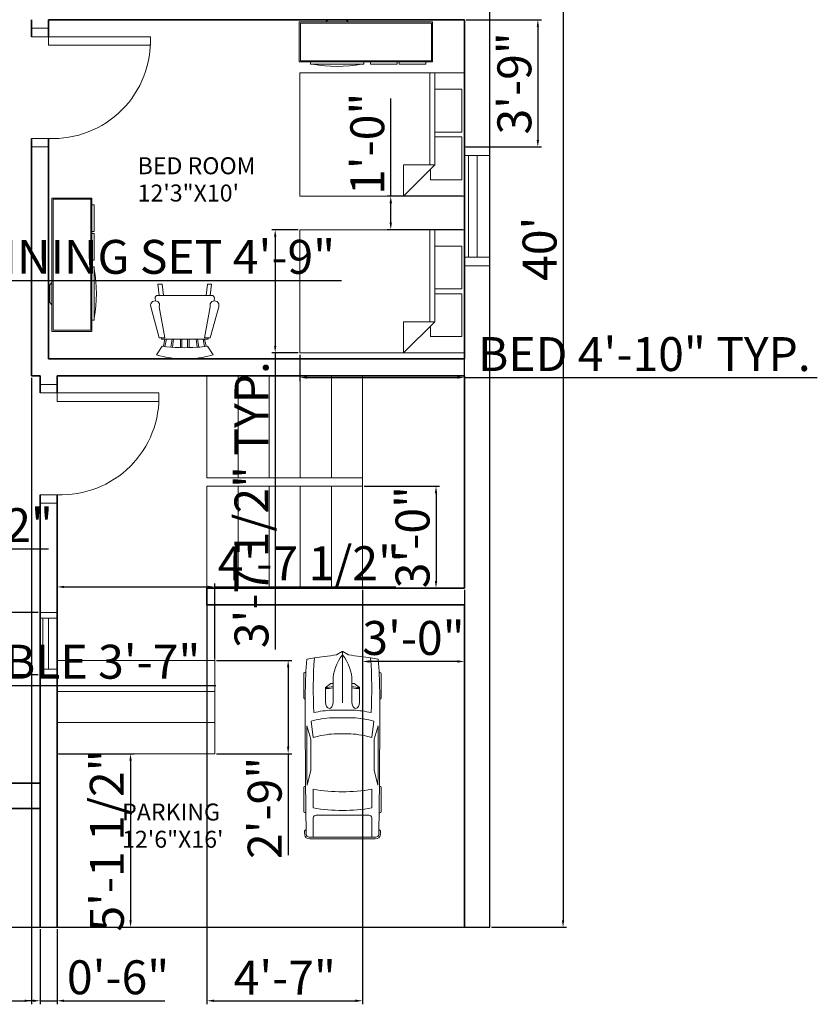
# Model space of a CAD drawing. Units: inches. Extents: x 2021 to 2692, y 429 to 1061.
# Tile 4 of 5: x 2362 to 2644, y 480 to 828. Entities that reach past the tile are written whole.
import ezdxf

# ---------------------------------------------------------------- set-up
doc = ezdxf.new("R2010")
doc.units = ezdxf.units.IN
for name, color, linetype, lineweight in [('A-ANNO-DIMS', 2, 'Continuous', 18), ('A-AREA-IDEN', 7, 'Continuous', 18), ('A-DOOR', 4, 'Continuous', 18), ('A-FLOR-STRS', 7, 'Continuous', 18), ('A-FURN', 8, 'Continuous', 13), ('A-GLAZ', 4, 'Continuous', 18), ('A-WALL', 7, 'Continuous', 35), ('C-PRKG-VEHI', 8, 'Continuous', 13), ('C-PROP', 3, 'Continuous', 25)]:
    doc.layers.add(name, color=color, linetype=linetype, lineweight=lineweight)
doc.styles.get("Standard").update_dxf_attribs({"font": 'arial.ttf'})
doc.dimstyles.new('ISO-25', dxfattribs={"dimtxt": 12, "dimasz": 2.5, "dimexe": 1.25, "dimexo": 0.625, "dimtad": 1, "dimdec": 0, "dimlunit": 3, "dimtxsty": 'Standard', "dimcen": 2.5, "dimadec": 0, "dimazin": 0, "dimtfac": 1, "dimtdec": 0, "dimtmove": 0, "dimatfit": 3, "dimfxl": 1, "dimarcsym": 0})

# ---------------------------------------------------------------- blocks, each defined once
blk = doc.blocks.new('Bed - Queen')
for p, q in [((0, -80.00003), (0, 0)), ((0, 0), (59.99999, 0)), ((59.99999, 0), (59.99999, -80.00003)), ((7.99999, -1.2), (28.79998, -1.2)), ((7.99999, -14.4), (7.99999, -1.2)), ((28.79998, -1.2), (28.79998, -14.4)), ((31.19999, -1.2), (51.99999, -1.2)), ((31.19999, -14.4), (31.19999, -1.2)), ((51.99999, -1.2), (51.99999, -16.4)), ((0, -14.4), (44.8, -14.4)), ((44.8, -16.8), (0, -16.8)), ((59.99999, -29.6), (44.8, -14.4)), ((44.8, -14.4), (44.8, -29.6)), ((51.99999, -16.4), (46.79936, -16.4)), ((44.8, -29.6), (59.99999, -29.6)), ((59.99999, -80.00003), (0, -80.00003))]:
    blk.add_line(p, q)
blk = doc.blocks.new('Entertainment Center')
for p, q in [((-4, 0), (-5, -1)), ((4, 0), (-4, 0)), ((5, -1), (4, 0)), ((-17, -19), (-17, -1)), ((-17, -1), (43, -1)), ((-16.5, -18.5), (-16.5, -1.5)), ((-16.5, -1.5), (42.5, -1.5)), ((42.5, -1.5), (42.5, -18.5)), ((43, -1), (43, -19)), ((43, -19), (-17, -19)), ((42.5, -18.5), (-16.5, -18.5)), ((-12, -20), (-12, -19)), ((12, -20), (-12, -20)), ((12, -19), (12, -20)), ((15, -20), (15, -19)), ((27, -20), (15, -20)), ((27, -19), (27, -20)), ((28, -20), (28, -19)), ((40, -20), (28, -20)), ((40, -19), (40, -20))]:
    blk.add_line(p, q)
blk.add_arc((0, 40), 61, 259.6111, 280.3889)
blk = doc.blocks.new('Chair - Rocking')
for p, q in [((-8, -4.5), (-10, -1.5)), ((8, -4.5), (10, -1.5)), ((-7.5, -4.5), (-7, -7)), ((-6.5, -7), (-7.02225, -4.43)), ((-4.5, -7), (-4.96674, -4.19951)), ((-4, -7), (-4.40532, -4.16272)), ((-1.5, -4.05012), (-1.5, -7)), ((-1, -7), (-1, -4.05012)), ((1, -7), (1, -4.04655)), ((1.5, -4.05012), (1.5, -7)), ((4, -7), (4.40187, -4.18694)), ((4.5, -7), (4.96761, -4.19437)), ((6.5, -7), (7, -4.4057)), ((7.5, -4.5), (7, -7)), ((-9, -7.5), (-12, -18.49999)), ((-7, -7.5), (-9, -7.5)), ((-9, -18.49999), (-7, -7.5)), ((-8.23428, -6.99939), (-8.3093, -7.47958)), ((-8.23041, -7), (8.23915, -7)), ((7, -7.5), (9, -7.5)), ((9, -18.49999), (7, -7.5)), ((8.31071, -7.48854), (8.23449, -7.00073)), ((9, -7.5), (12, -18.49999)), ((-10.36644, -20.64523), (-10.5, -21.49999)), ((10.5, -21.49999), (10.3575, -20.58798)), ((-9, -22.49999), (-9.5, -26.49999)), ((0, -22.49999), (-9.5, -22.49999)), ((-8, -26.49999), (-7.5, -22.49999)), ((0, -22.49999), (9.5, -22.49999)), ((8, -26.49999), (7.5, -22.49999)), ((9, -22.49999), (9.5, -26.49999)), ((-9.5, -26.49999), (-8, -26.49999)), ((9.5, -26.49999), (8, -26.49999))]:
    blk.add_line(p, q)
for centre, radius, start, end in [((0, -34.08333), 34.08333, 72.93847, 107.0615), ((0, -68.25004), 64.25, 93.92211, 97.15267), ((0, -68.25004), 64.25, 82.84733, 93.92211), ((-10.5, -18.99999), 1.58114, 161.5651, 18.43495), ((10.5, -18.99999), 1.58114, 161.5651, 18.43495), ((-9.5, -21.49999), 1, 180, 270), ((9.5, -21.49999), 1, 270, 0)]:
    blk.add_arc(centre, radius, start, end)
blk = doc.blocks.new('*U14')
for p, q in [((21.1, 37.41), (21.1, 36.83)), ((46.55, 38.89), (22.35, 38.89)), ((47.8, 37.39), (47.8, 37.41)), ((70.03, 31.54), (86.41, 29.35)), ((87.99, 31.87), (74.76, 35.92)), ((134.31, 35.6), (119.29, 31.78)), ((135.45, 37.07), (135.45, 37.41)), ((136.7, 38.89), (160.9, 38.89)), ((162.15, 37.41), (162.15, 36.77)), ((186.47, -33.5), (186.47, 33.5)), ((188.4, -32.76), (188.4, 32.76)), ((138.42, 29.35), (157.25, 29.35)), ((164.52, 26.39), (164.52, -26.39)), ((186.47, 29.35), (167.01, 29.35)), ((32.12, 9.51), (32.12, 11.15)), ((32.27, 11.63), (36.13, 17.17)), ((36.13, 17.17), (50.94, 17.17)), ((58.92, -10.77), (58.92, 10.77)), ((66.55, -10.53), (66.55, 10.53)), ((186.47, -10.53), (186.47, 10.53)), ((3.27, 6.13), (0.1, 0.41)), ((29.77, 9.51), (51.68, 9.51)), ((82.74, 8.5), (82.74, -8.5)), ((0, 0), (51.68, 0)), ((0.1, -0.41), (3.27, -6.13)), ((29.77, -9.51), (51.68, -9.51)), ((32.12, -9.51), (32.12, -11.15)), ((32.27, -11.63), (36.13, -17.17)), ((36.13, -17.17), (50.94, -17.17)), ((86.41, -29.35), (70.03, -31.54)), ((157.25, -29.35), (138.42, -29.35)), ((167.01, -29.35), (186.47, -29.35)), ((21.1, -37.41), (21.1, -36.83)), ((46.55, -38.89), (22.35, -38.89)), ((47.8, -37.39), (47.8, -37.41)), ((87.99, -31.87), (74.76, -35.92)), ((134.31, -35.6), (119.29, -31.78)), ((135.45, -37.07), (135.45, -37.41)), ((136.7, -38.89), (160.9, -38.89)), ((162.15, -37.41), (162.15, -36.77))]:
    blk.add_line(p, q)
for centre, major_axis, ratio, start_param, end_param in [((266.03, -27.52), (0, 313.31), 0.842304, 1.367076, 1.39176), ((37.47, -593.96), (0, -623.33), 0.842304, 3.096046, 3.200911), ((41.19, -490.86), (0, 528.23), 0.842304, 0.00281, 0.075598), ((22.35, 37.41), (0, -1.48), 0.842304, 3.141593, 4.712389), ((64.48, -10555.62), (0, 10593.03), 0.842304, -0.013397, 0.002797), ((46.55, 37.41), (0, 1.48), 0.842304, -1.570796, 0), ((135.29, 5.39), (0, 81.77), 0.842304, 1.245306, 1.50788), ((64.48, -10555.62), (0, -10591.55), 0.842304, 3.133765, 3.140441), ((95.79, -3666.35), (0, -3698.24), 0.842304, 3.134049, 3.144098), ((136.7, 37.41), (0, -1.48), 0.842304, 3.141593, 4.712389), ((160.9, 37.41), (0, 1.48), 0.842304, -1.570796, 0), ((180.63, 35.84), (0, 2.22), 0.842304, -0.013017, 1.249894), ((64.48, -10556.36), (0, 10595.31), 0.842304, -0.013397, -0.013017), ((183.98, 33.5), (0, -2.96), 0.842304, 1.570796, 3.128196), ((183.98, 32.76), (0, -5.25), 0.842304, 1.570796, 3.128196), ((259.18, -27.52), (0, -305.3), 0.842304, 4.528606, 4.561838), ((134.4, 5.39), (0, -89.78), 0.842304, 4.449482, 4.652344), ((149.6, 2.8), (0, -79.58), 0.842304, 4.372215, 4.640744), ((17.08, 0), (0, 147.02), 0.842304, 4.511394, 4.913384), ((35.91, 0), (0, 147.02), 0.842304, 4.511394, 4.913384), ((167.01, 26.39), (0, 2.96), 0.842304, 0, 1.570796), ((-204.49, 52.4), (0, -250.96), 0.842304, 1.385369, 1.434372), ((32.75, 11.15), (0, 0.74), 0.842304, 0.879714, 1.570796), ((13.04, 17.01), (0, 27.42), 0.842304, 4.435146, 4.718221), ((14.2, 17.01), (0, 27.42), 0.842304, 4.435146, 4.718221), ((50.79, 13.34), (6.34, -0.36), 0.603834, -1.395552, 1.581315), ((0.62, 0), (0, -0.74), 0.842304, 4.131459, 5.293319), ((29.77, -46.66), (0, 56.17), 0.842304, 0, 0.590319), ((-204.49, -52.4), (0, 250.96), 0.842304, -1.434372, -1.385369), ((29.77, 46.66), (0, 56.17), 0.842304, 2.551274, 3.141593), ((13.04, -17.01), (0, -27.42), 0.842304, 1.564964, 1.848039), ((14.2, -17.01), (0, -27.42), 0.842304, 1.564964, 1.848039), ((149.6, -2.8), (0, -79.58), 0.842304, -1.499151, -1.230623), ((259.18, 27.52), (0, 305.3), 0.842304, 1.721348, 1.754579), ((32.75, -11.15), (0, -0.74), 0.842304, 4.712389, 5.403472), ((134.4, -5.39), (0, -89.78), 0.842304, -1.510751, -1.307889), ((135.29, -5.39), (0, -81.77), 0.842304, -1.50788, -1.245306), ((266.03, 27.52), (0, 313.31), 0.842304, 1.749832, 1.774517), ((37.47, 593.96), (0, -623.33), 0.842304, -0.059319, 0.045547), ((167.01, -26.39), (0, -2.96), 0.842304, 4.712389, 6.283185), ((41.19, 490.86), (0, -528.23), 0.842304, -0.075598, -0.00281), ((22.35, -37.41), (0, 1.48), 0.842304, 1.570796, 3.141593), ((64.48, 10555.62), (0, 10593.03), 0.842304, 3.138796, 3.15499), ((46.55, -37.41), (0, -1.48), 0.842304, 0, 1.570796), ((64.48, 10555.62), (0, -10591.55), 0.842304, 0.001152, 0.007828), ((95.79, 3666.35), (0, -3698.24), 0.842304, -0.002505, 0.007544), ((136.7, -37.41), (0, -1.48), 0.842304, -1.570796, 0), ((160.9, -37.41), (0, 1.48), 0.842304, 3.141593, 4.712389), ((180.63, -35.84), (0, -2.22), 0.842304, -1.249894, 0.013017), ((64.48, 10556.36), (0, 10595.31), 0.842304, 3.15461, 3.15499), ((183.98, -33.5), (0, 2.96), 0.842304, 3.15499, 4.712389), ((183.98, -32.76), (0, -5.25), 0.842304, 0.013397, 1.570796)]:
    blk.add_ellipse(centre, major_axis=major_axis, ratio=ratio, start_param=start_param, end_param=end_param)
at = {"extrusion": (0, 0, -1)}
blk.add_ellipse((50.79, -13.34), major_axis=(6.34, 0.36), ratio=0.603834, start_param=-1.395552, end_param=1.581315, dxfattribs=at)
blk = doc.blocks.new('*D16')
at = {"layer": 'A-ANNO-DIMS', "color": 0, "lineweight": -2, "transparency": 16777216}
for p, q in [((2528.73, 986.96), (2555.26, 986.96)), ((2554.01, 984.46), (2554.01, 509.46)), ((2528.73, 506.96), (2555.26, 506.96))]:
    blk.add_line(p, q, dxfattribs=at)
at = {"layer": 'A-ANNO-DIMS', "color": 0, "transparency": 16777216}
for points in [[(2553.59, 984.46), (2554.43, 984.46), (2554.01, 986.96)], [(2553.59, 509.46), (2554.43, 509.46), (2554.01, 506.96)]]:
    blk.add_solid(points, dxfattribs=at)
at = {"layer": 'Defpoints', "color": 0, "transparency": 16777216}
for p in [(2528.11, 986.96), (2528.11, 506.96), (2554.01, 506.96)]:
    blk.add_point(p, dxfattribs=at)
at = {"layer": 'A-ANNO-DIMS', "color": 0, "transparency": 16777216, "insert": (2547.26, 746.96), "char_height": 12, "attachment_point": 5, "rotation": 90}
blk.add_mtext("40'", dxfattribs=at)
blk = doc.blocks.new('DOOR-SWING-36IN')
for p, q in [((36.03, 42), (42.03, 42)), ((36.03, 39), (42.03, 39)), ((36.03, 3), (42.03, 3)), ((36.03, 0), (42.03, 0))]:
    blk.add_line(p, q)
blk.add_lwpolyline([(36.03, 39), (0.03, 39), (0.03, 36), (36.03, 36)], close=True)
blk.add_arc((34.53, 37.5), 34.53, 177.5104, 272.4896)
blk = doc.blocks.new('WIN-36IN')
for p, q in [((0, 0), (0, 9)), ((3, 9), (39, 9)), ((3, 0), (3, 9)), ((3, 7.5), (39, 7.5)), ((39, 9), (39, 0)), ((42, 9), (42, 0)), ((3, 4.5), (39, 4.5)), ((39, 0), (3, 0))]:
    blk.add_line(p, q)
blk = doc.blocks.new('*D28')
at = {"layer": 'A-ANNO-DIMS', "color": 0, "lineweight": -2, "transparency": 16777216}
for p, q in [((2460.96, 709.49), (2460.96, 700.15)), ((2519.08, 709.49), (2519.08, 700.15)), ((2463.46, 701.4), (2516.58, 701.4)), ((2519.08, 701.4), (2643.89, 701.4))]:
    blk.add_line(p, q, dxfattribs=at)
at = {"layer": 'A-ANNO-DIMS', "color": 0, "transparency": 16777216}
for points in [[(2463.46, 701.81), (2463.46, 700.98), (2460.96, 701.4)], [(2516.58, 701.81), (2516.58, 700.98), (2519.08, 701.4)]]:
    blk.add_solid(points, dxfattribs=at)
at = {"layer": 'Defpoints', "color": 0, "transparency": 16777216}
for p in [(2460.96, 710.11), (2519.08, 710.11), (2519.08, 701.4)]:
    blk.add_point(p, dxfattribs=at)
at = {"layer": 'A-ANNO-DIMS', "color": 0, "transparency": 16777216, "insert": (2582.73, 708.15), "char_height": 12, "attachment_point": 5}
blk.add_mtext('BED 4\'-10" TYP.', dxfattribs=at)
blk = doc.blocks.new('*D29')
at = {"layer": 'A-ANNO-DIMS', "color": 0, "lineweight": -2, "transparency": 16777216}
for p, q in [((2460.33, 753.7), (2450.99, 753.7)), ((2452.24, 751.2), (2452.24, 712.61)), ((2460.33, 710.11), (2450.99, 710.11)), ((2452.24, 710.11), (2452.24, 605.27))]:
    blk.add_line(p, q, dxfattribs=at)
at = {"layer": 'A-ANNO-DIMS', "color": 0, "transparency": 16777216}
for points in [[(2451.82, 751.2), (2452.65, 751.2), (2452.24, 753.7)], [(2451.82, 712.61), (2452.65, 712.61), (2452.24, 710.11)]]:
    blk.add_solid(points, dxfattribs=at)
at = {"layer": 'Defpoints', "color": 0, "transparency": 16777216}
for p in [(2460.96, 753.7), (2452.24, 710.11), (2460.96, 710.11)]:
    blk.add_point(p, dxfattribs=at)
at = {"layer": 'A-ANNO-DIMS', "color": 0, "transparency": 16777216, "insert": (2445.4, 656.44), "char_height": 12, "attachment_point": 5, "rotation": 90}
blk.add_mtext('3\'-7 1/2" TYP.', dxfattribs=at)
blk = doc.blocks.new('*D38')
at = {"layer": 'A-ANNO-DIMS', "color": 0, "lineweight": -2, "transparency": 16777216}
for p, q in [((2283.11, 743.62), (2283.11, 734.45)), ((2340.09, 743.62), (2340.09, 734.45)), ((2285.61, 735.7), (2337.59, 735.7)), ((2340.09, 735.7), (2475.73, 735.7))]:
    blk.add_line(p, q, dxfattribs=at)
at = {"layer": 'A-ANNO-DIMS', "color": 0, "transparency": 16777216}
for points in [[(2285.61, 736.12), (2285.61, 735.28), (2283.11, 735.7)], [(2337.59, 736.12), (2337.59, 735.28), (2340.09, 735.7)]]:
    blk.add_solid(points, dxfattribs=at)
at = {"layer": 'Defpoints', "color": 0, "transparency": 16777216}
for p in [(2283.11, 744.25), (2340.09, 744.25), (2340.09, 735.7)]:
    blk.add_point(p, dxfattribs=at)
at = {"layer": 'A-ANNO-DIMS', "color": 0, "transparency": 16777216, "insert": (2409.16, 742.53), "char_height": 12, "attachment_point": 5}
blk.add_mtext('DINING SET 4\'-9"', dxfattribs=at)
blk = doc.blocks.new('*D47')
at = {"layer": 'A-ANNO-DIMS', "color": 0, "lineweight": -2, "transparency": 16777216}
for p, q in [((2278.74, 634.19), (2278.74, 642.06)), ((2281.24, 640.81), (2305.76, 640.81)), ((2308.26, 634.19), (2308.26, 642.06)), ((2308.26, 640.81), (2372.08, 640.81))]:
    blk.add_line(p, q, dxfattribs=at)
at = {"layer": 'A-ANNO-DIMS', "color": 0, "transparency": 16777216}
for points in [[(2281.24, 641.23), (2281.24, 640.4), (2278.74, 640.81)], [(2305.76, 641.23), (2305.76, 640.4), (2308.26, 640.81)]]:
    blk.add_solid(points, dxfattribs=at)
at = {"layer": 'Defpoints', "color": 0, "transparency": 16777216}
for p in [(2308.26, 640.81), (2278.74, 633.57), (2308.26, 633.57)]:
    blk.add_point(p, dxfattribs=at)
at = {"layer": 'A-ANNO-DIMS', "color": 0, "transparency": 16777216, "insert": (2341.42, 647.64), "char_height": 12, "attachment_point": 5}
blk.add_mtext('2\'-5 1/2"', dxfattribs=at)
blk = doc.blocks.new('*D48')
at = {"layer": 'A-ANNO-DIMS', "color": 0, "lineweight": -2, "transparency": 16777216}
for p, q in [((2222.09, 598.36), (2222.09, 591.25)), ((2265.33, 598.36), (2265.33, 591.25)), ((2224.59, 592.5), (2262.83, 592.5)), ((2265.33, 592.5), (2431.25, 592.5))]:
    blk.add_line(p, q, dxfattribs=at)
at = {"layer": 'A-ANNO-DIMS', "color": 0, "transparency": 16777216}
for points in [[(2224.59, 592.92), (2224.59, 592.08), (2222.09, 592.5)], [(2262.83, 592.92), (2262.83, 592.08), (2265.33, 592.5)]]:
    blk.add_solid(points, dxfattribs=at)
at = {"layer": 'Defpoints', "color": 0, "transparency": 16777216}
for p in [(2222.09, 598.99), (2265.33, 598.99), (2265.33, 592.5)]:
    blk.add_point(p, dxfattribs=at)
at = {"layer": 'A-ANNO-DIMS', "color": 0, "transparency": 16777216, "insert": (2349.54, 599.34), "char_height": 12, "attachment_point": 5}
blk.add_mtext('COFFEE TABLE 3\'-7"', dxfattribs=at)
blk = doc.blocks.new('*D55')
at = {"layer": 'A-ANNO-DIMS', "color": 0, "lineweight": -2, "transparency": 16777216}
for p, q in [((2369.11, 506.34), (2369.11, 479.73)), ((2375.11, 506.34), (2375.11, 479.73)), ((2366.61, 480.98), (2364.11, 480.98)), ((2369.11, 480.98), (2375.11, 480.98)), ((2377.61, 480.98), (2413.26, 480.98))]:
    blk.add_line(p, q, dxfattribs=at)
at = {"layer": 'A-ANNO-DIMS', "color": 0, "transparency": 16777216}
for points in [[(2366.61, 481.4), (2366.61, 480.56), (2369.11, 480.98)], [(2377.61, 481.4), (2377.61, 480.56), (2375.11, 480.98)]]:
    blk.add_solid(points, dxfattribs=at)
at = {"layer": 'Defpoints', "color": 0, "transparency": 16777216}
for p in [(2369.11, 506.96), (2375.11, 506.96), (2375.11, 480.98)]:
    blk.add_point(p, dxfattribs=at)
at = {"layer": 'A-ANNO-DIMS', "color": 0, "transparency": 16777216, "insert": (2396.68, 487.73), "char_height": 12, "attachment_point": 5}
blk.add_mtext('0\'-6"', dxfattribs=at)
blk = doc.blocks.new('*D56')
at = {"layer": 'A-ANNO-DIMS', "color": 0, "lineweight": -2, "transparency": 16777216}
for p, q in [((2375.11, 601.99), (2375.11, 628.6)), ((2377.61, 627.35), (2428.34, 627.35)), ((2430.84, 601.99), (2430.84, 628.6)), ((2430.84, 627.35), (2494.93, 627.35))]:
    blk.add_line(p, q, dxfattribs=at)
at = {"layer": 'A-ANNO-DIMS', "color": 0, "transparency": 16777216}
for points in [[(2377.61, 627.77), (2377.61, 626.94), (2375.11, 627.35)], [(2428.34, 627.77), (2428.34, 626.94), (2430.84, 627.35)]]:
    blk.add_solid(points, dxfattribs=at)
at = {"layer": 'Defpoints', "color": 0, "transparency": 16777216}
for p in [(2430.84, 627.35), (2375.11, 601.37), (2430.84, 601.37)]:
    blk.add_point(p, dxfattribs=at)
at = {"layer": 'A-ANNO-DIMS', "color": 0, "transparency": 16777216, "insert": (2464.13, 634.18), "char_height": 12, "attachment_point": 5}
blk.add_mtext('4\'-7 1/2"', dxfattribs=at)
blk = doc.blocks.new('*D57')
at = {"layer": 'A-ANNO-DIMS', "color": 0, "lineweight": -2, "transparency": 16777216}
for p, q in [((2431.46, 601.37), (2458.07, 601.37)), ((2456.82, 598.87), (2456.82, 570.87)), ((2431.46, 568.37), (2458.07, 568.37)), ((2456.82, 568.37), (2456.82, 532.52))]:
    blk.add_line(p, q, dxfattribs=at)
at = {"layer": 'A-ANNO-DIMS', "color": 0, "transparency": 16777216}
for points in [[(2456.41, 598.87), (2457.24, 598.87), (2456.82, 601.37)], [(2456.41, 570.87), (2457.24, 570.87), (2456.82, 568.37)]]:
    blk.add_solid(points, dxfattribs=at)
at = {"layer": 'Defpoints', "color": 0, "transparency": 16777216}
for p in [(2430.84, 601.37), (2430.84, 568.37), (2456.82, 568.37)]:
    blk.add_point(p, dxfattribs=at)
at = {"layer": 'A-ANNO-DIMS', "color": 0, "transparency": 16777216, "insert": (2450.07, 549.19), "char_height": 12, "attachment_point": 5, "rotation": 90}
blk.add_mtext('2\'-9"', dxfattribs=at)
blk = doc.blocks.new('*D58')
at = {"layer": 'A-ANNO-DIMS', "color": 0, "lineweight": -2, "transparency": 16777216}
for p, q in [((2483.73, 662.96), (2510.34, 662.96)), ((2509.09, 660.46), (2509.09, 629.46)), ((2483.73, 626.96), (2510.34, 626.96))]:
    blk.add_line(p, q, dxfattribs=at)
at = {"layer": 'A-ANNO-DIMS', "color": 0, "transparency": 16777216}
for points in [[(2508.68, 660.46), (2509.51, 660.46), (2509.09, 662.96)], [(2508.68, 629.46), (2509.51, 629.46), (2509.09, 626.96)]]:
    blk.add_solid(points, dxfattribs=at)
at = {"layer": 'Defpoints', "color": 0, "transparency": 16777216}
for p in [(2483.11, 662.96), (2483.11, 626.96), (2509.09, 626.96)]:
    blk.add_point(p, dxfattribs=at)
at = {"layer": 'A-ANNO-DIMS', "color": 0, "transparency": 16777216, "insert": (2502.34, 644.96), "char_height": 12, "attachment_point": 5, "rotation": 90}
blk.add_mtext('3\'-0"', dxfattribs=at)
blk = doc.blocks.new('*D59')
at = {"layer": 'A-ANNO-DIMS', "color": 0, "lineweight": -2, "transparency": 16777216}
for p, q in [((2428.11, 626.34), (2428.11, 479.73)), ((2483.11, 626.34), (2483.11, 479.73)), ((2430.61, 480.98), (2480.61, 480.98))]:
    blk.add_line(p, q, dxfattribs=at)
at = {"layer": 'A-ANNO-DIMS', "color": 0, "transparency": 16777216}
for points in [[(2430.61, 481.4), (2430.61, 480.56), (2428.11, 480.98)], [(2480.61, 481.4), (2480.61, 480.56), (2483.11, 480.98)]]:
    blk.add_solid(points, dxfattribs=at)
at = {"layer": 'Defpoints', "color": 0, "transparency": 16777216}
for p in [(2428.11, 626.96), (2483.11, 626.96), (2483.11, 480.98)]:
    blk.add_point(p, dxfattribs=at)
at = {"layer": 'A-ANNO-DIMS', "color": 0, "transparency": 16777216, "insert": (2455.61, 487.6), "char_height": 12, "attachment_point": 5}
blk.add_mtext('4\'-7"', dxfattribs=at)
blk = doc.blocks.new('*D60')
at = {"layer": 'A-ANNO-DIMS', "color": 0, "lineweight": -2, "transparency": 16777216}
for p, q in [((2483.11, 626.34), (2483.11, 599.73)), ((2519.11, 626.34), (2519.11, 599.73)), ((2516.61, 600.98), (2485.61, 600.98))]:
    blk.add_line(p, q, dxfattribs=at)
at = {"layer": 'A-ANNO-DIMS', "color": 0, "transparency": 16777216}
for points in [[(2485.61, 601.4), (2485.61, 600.56), (2483.11, 600.98)], [(2516.61, 601.4), (2516.61, 600.56), (2519.11, 600.98)]]:
    blk.add_solid(points, dxfattribs=at)
at = {"layer": 'Defpoints', "color": 0, "transparency": 16777216}
for p in [(2483.11, 626.96), (2519.11, 626.96), (2483.11, 600.98)]:
    blk.add_point(p, dxfattribs=at)
at = {"layer": 'A-ANNO-DIMS', "color": 0, "transparency": 16777216, "insert": (2501.11, 607.74), "char_height": 12, "attachment_point": 5}
blk.add_mtext('3\'-0"', dxfattribs=at)
blk = doc.blocks.new('*D61')
at = {"layer": 'A-ANNO-DIMS', "color": 0, "lineweight": -2, "transparency": 16777216}
for p, q in [((2375.73, 568.37), (2402.34, 568.37)), ((2401.09, 565.87), (2401.09, 509.46)), ((2375.73, 506.96), (2402.34, 506.96))]:
    blk.add_line(p, q, dxfattribs=at)
at = {"layer": 'A-ANNO-DIMS', "color": 0, "transparency": 16777216}
for points in [[(2400.68, 565.87), (2401.51, 565.87), (2401.09, 568.37)], [(2400.68, 509.46), (2401.51, 509.46), (2401.09, 506.96)]]:
    blk.add_solid(points, dxfattribs=at)
at = {"layer": 'Defpoints', "color": 0, "transparency": 16777216}
for p in [(2375.11, 568.37), (2375.11, 506.96), (2401.09, 506.96)]:
    blk.add_point(p, dxfattribs=at)
at = {"layer": 'A-ANNO-DIMS', "color": 0, "transparency": 16777216, "insert": (2394.27, 537.67), "char_height": 12, "attachment_point": 5, "rotation": 90}
blk.add_mtext('5\'-1 1/2"', dxfattribs=at)
blk = doc.blocks.new('*D64')
at = {"layer": 'A-ANNO-DIMS', "color": 0, "lineweight": -2, "transparency": 16777216}
for p, q in [((2519.73, 827.96), (2546.34, 827.96)), ((2545.09, 825.46), (2545.09, 785.44)), ((2519.73, 782.94), (2546.34, 782.94))]:
    blk.add_line(p, q, dxfattribs=at)
at = {"layer": 'A-ANNO-DIMS', "color": 0, "transparency": 16777216}
for points in [[(2544.68, 825.46), (2545.51, 825.46), (2545.09, 827.96)], [(2544.68, 785.44), (2545.51, 785.44), (2545.09, 782.94)]]:
    blk.add_solid(points, dxfattribs=at)
at = {"layer": 'Defpoints', "color": 0, "transparency": 16777216}
for p in [(2519.11, 827.96), (2519.11, 782.94), (2545.09, 782.94)]:
    blk.add_point(p, dxfattribs=at)
at = {"layer": 'A-ANNO-DIMS', "color": 0, "transparency": 16777216, "insert": (2538.34, 805.45), "char_height": 12, "attachment_point": 5, "rotation": 90}
blk.add_mtext('3\'-9"', dxfattribs=at)
blk = doc.blocks.new('*D68')
at = {"layer": 'A-ANNO-DIMS', "color": 0, "lineweight": -2, "transparency": 16777216}
for p, q in [((2299.94, 701.34), (2299.94, 479.73)), ((2366.11, 701.34), (2366.11, 479.73)), ((2302.44, 480.98), (2363.61, 480.98))]:
    blk.add_line(p, q, dxfattribs=at)
at = {"layer": 'A-ANNO-DIMS', "color": 0, "transparency": 16777216}
for points in [[(2302.44, 481.4), (2302.44, 480.56), (2299.94, 480.98)], [(2363.61, 481.4), (2363.61, 480.56), (2366.11, 480.98)]]:
    blk.add_solid(points, dxfattribs=at)
at = {"layer": 'Defpoints', "color": 0, "transparency": 16777216}
for p in [(2299.94, 701.96), (2366.11, 701.96), (2366.11, 480.98)]:
    blk.add_point(p, dxfattribs=at)
at = {"layer": 'A-ANNO-DIMS', "color": 0, "transparency": 16777216, "insert": (2333.02, 487.73), "char_height": 12, "attachment_point": 5}
blk.add_mtext('5\'-6"', dxfattribs=at)
blk = doc.blocks.new('*D69')
at = {"layer": 'A-ANNO-DIMS', "color": 0, "lineweight": -2, "transparency": 16777216}
for p, q in [((2142.12, 596.25), (2142.12, 659.85)), ((2368.48, 596.25), (2140.87, 596.25)), ((2142.12, 560.46), (2142.12, 593.75)), ((2368.48, 557.96), (2140.87, 557.96))]:
    blk.add_line(p, q, dxfattribs=at)
at = {"layer": 'A-ANNO-DIMS', "color": 0, "transparency": 16777216}
for points in [[(2141.71, 593.75), (2142.54, 593.75), (2142.12, 596.25)], [(2141.71, 560.46), (2142.54, 560.46), (2142.12, 557.96)]]:
    blk.add_solid(points, dxfattribs=at)
at = {"layer": 'Defpoints', "color": 0, "transparency": 16777216}
for p in [(2142.12, 596.25), (2369.11, 596.25), (2369.11, 557.96)]:
    blk.add_point(p, dxfattribs=at)
at = {"layer": 'A-ANNO-DIMS', "color": 0, "transparency": 16777216, "insert": (2135.29, 629.3), "char_height": 12, "attachment_point": 5, "rotation": 90}
blk.add_mtext('3\'-2 1/2"', dxfattribs=at)
blk = doc.blocks.new('*D70')
at = {"layer": 'A-ANNO-DIMS', "color": 0, "lineweight": -2, "transparency": 16777216}
for p, q in [((2142.12, 618.25), (2142.12, 662.09)), ((2368.48, 618.25), (2140.87, 618.25)), ((2142.12, 598.75), (2142.12, 615.75)), ((2368.48, 596.25), (2140.87, 596.25))]:
    blk.add_line(p, q, dxfattribs=at)
at = {"layer": 'A-ANNO-DIMS', "color": 0, "transparency": 16777216}
for points in [[(2141.71, 615.75), (2142.54, 615.75), (2142.12, 618.25)], [(2141.71, 598.75), (2142.54, 598.75), (2142.12, 596.25)]]:
    blk.add_solid(points, dxfattribs=at)
at = {"layer": 'Defpoints', "color": 0, "transparency": 16777216}
for p in [(2142.12, 618.25), (2369.11, 618.25), (2369.11, 596.25)]:
    blk.add_point(p, dxfattribs=at)
at = {"layer": 'A-ANNO-DIMS', "color": 0, "transparency": 16777216, "insert": (2135.37, 641.42), "char_height": 12, "attachment_point": 5, "rotation": 90}
blk.add_mtext('1\'-10"', dxfattribs=at)
blk = doc.blocks.new('*D72')
at = {"layer": 'A-ANNO-DIMS', "color": 0, "lineweight": -2, "transparency": 16777216}
for p, q in [((2493.09, 765.57), (2493.09, 800.09)), ((2518.45, 765.57), (2491.84, 765.57)), ((2493.09, 756.2), (2493.09, 763.07)), ((2518.45, 753.7), (2491.84, 753.7))]:
    blk.add_line(p, q, dxfattribs=at)
at = {"layer": 'A-ANNO-DIMS', "color": 0, "transparency": 16777216}
for points in [[(2492.67, 763.07), (2493.51, 763.07), (2493.09, 765.57)], [(2492.67, 756.2), (2493.51, 756.2), (2493.09, 753.7)]]:
    blk.add_solid(points, dxfattribs=at)
at = {"layer": 'Defpoints', "color": 0, "transparency": 16777216}
for p in [(2493.09, 765.57), (2519.08, 765.57), (2519.08, 753.7)]:
    blk.add_point(p, dxfattribs=at)
at = {"layer": 'A-ANNO-DIMS', "color": 0, "transparency": 16777216, "insert": (2486.34, 784.08), "char_height": 12, "attachment_point": 5, "rotation": 90}
blk.add_mtext('1\'-0"', dxfattribs=at)

msp = doc.modelspace()

# ---------------------------------------------------------------- linework, layer by layer
at = {"layer": 'A-DOOR'}
for p, q in [((2372.11, 824.96), (2366.11, 824.96)), ((2372.11, 821.96), (2366.11, 821.96)), ((2372.11, 785.96), (2366.11, 785.96)), ((2372.11, 782.96), (2366.11, 782.96))]:
    msp.add_line(p, q, dxfattribs=at)
msp.add_lwpolyline([(2372.11, 818.96), (2408.11, 818.96), (2408.11, 821.96), (2372.11, 821.96)], close=True, dxfattribs=at)
msp.add_arc((2373.61, 820.46), 34.53, 267.5104, 2.4896, dxfattribs=at)
at = {"layer": 'A-FLOR-STRS'}
for p, q in [((2428.11, 665.96), (2428.11, 701.96)), ((2439.11, 665.96), (2439.11, 701.96)), ((2450.11, 665.96), (2450.11, 701.96)), ((2461.11, 665.96), (2461.11, 701.96)), ((2472.11, 665.96), (2472.11, 701.96)), ((2483.11, 626.96), (2483.11, 701.96)), ((2483.11, 665.96), (2428.11, 665.96)), ((2483.11, 662.96), (2428.11, 662.96)), ((2428.11, 626.96), (2428.11, 662.96)), ((2439.11, 626.96), (2439.11, 662.96)), ((2450.11, 626.96), (2450.11, 662.96)), ((2461.11, 626.96), (2461.11, 662.96)), ((2472.11, 626.96), (2472.11, 662.96)), ((2430.84, 620.96), (2430.84, 568.37)), ((2430.84, 601.37), (2375.11, 601.37)), ((2430.84, 590.37), (2375.11, 590.37)), ((2430.84, 579.37), (2375.11, 579.37)), ((2430.84, 568.37), (2375.11, 568.37))]:
    msp.add_line(p, q, dxfattribs=at)
at = {"layer": 'A-GLAZ'}
for p, q in [((2375.11, 618.25), (2369.11, 618.25)), ((2375.11, 616.25), (2369.11, 616.25)), ((2369.11, 616.25), (2369.11, 598.25)), ((2370.11, 598.25), (2370.11, 616.25)), ((2372.11, 598.25), (2372.11, 616.25)), ((2375.11, 598.25), (2375.11, 616.25)), ((2369.11, 598.25), (2375.11, 598.25)), ((2369.11, 596.25), (2375.11, 596.25))]:
    msp.add_line(p, q, dxfattribs=at)
at = {"layer": 'A-WALL'}
for p, q in [((2366.11, 821.96), (2366.11, 827.96)), ((2519.11, 827.96), (2372.11, 827.96)), ((2372.11, 821.96), (2372.11, 827.96)), ((2519.11, 707.96), (2519.11, 827.96)), ((2366.11, 707.96), (2366.11, 785.96)), ((2372.11, 707.96), (2372.11, 785.96)), ((2366.11, 707.96), (2366.11, 701.96)), ((2519.11, 707.96), (2372.11, 707.96)), ((2369.11, 701.96), (2366.11, 701.96)), ((2369.11, 695.96), (2369.11, 701.96)), ((2519.11, 701.96), (2375.11, 701.96)), ((2375.11, 695.96), (2375.11, 701.96)), ((2519.11, 626.96), (2519.11, 701.96)), ((2369.11, 548.96), (2369.11, 659.96)), ((2375.11, 626.96), (2375.11, 659.96)), ((2375.11, 626.96), (2375.11, 620.96)), ((2519.11, 626.96), (2428.11, 626.96)), ((2428.11, 626.96), (2428.11, 620.96)), ((2375.11, 515.96), (2375.11, 620.96)), ((2519.11, 620.96), (2428.11, 620.96)), ((2519.11, 506.96), (2519.11, 620.96)), ((2369.11, 557.96), (2177.11, 557.96)), ((2369.11, 515.96), (2369.11, 551.96)), ((2369.11, 548.96), (2168.11, 548.96)), ((2369.11, 515.96), (2369.11, 506.96)), ((2375.11, 515.96), (2375.11, 506.96))]:
    msp.add_line(p, q, dxfattribs=at)
at = {"layer": 'C-PROP'}
msp.add_lwpolyline([(2168.11, 506.96), (2528.11, 506.96), (2528.11, 986.96), (2168.11, 986.96)], close=True, dxfattribs=at)

# ---------------------------------------------------------------- block references
at = {"layer": 'A-DOOR', "extrusion": (0, 0, -1), "zscale": -1}
msp.add_blockref('DOOR-SWING-36IN', (-2411.14, 656.96), dxfattribs=at)
at = {"layer": 'A-FURN', "xscale": 0.7857640072773148, "yscale": 0.7857640072773148, "zscale": 0.7857640072773148}
msp.add_blockref('Entertainment Center', (2474.11, 827.96), dxfattribs=at)
at = {"layer": 'A-FURN'}
for name, p, xscale, yscale, zscale, rotation in [('Bed - Queen', (2519.08, 809.16), 0.7264929112576234, 0.7264929112576234, 0.7264929112576234, 270), ('Entertainment Center', (2372.5, 731.09), 0.7857640072773148, 0.7857640072773148, 0.7857640072773148, 90), ('Bed - Queen', (2519.08, 753.7), 0.7264929112576234, 0.7264929112576234, 0.7264929112576234, 270)]:
    msp.add_blockref(name, p, dxfattribs=dict(at, xscale=xscale, yscale=yscale, zscale=zscale, rotation=rotation))
at = {"layer": 'A-FURN', "rotation": 180}
msp.add_blockref('Chair - Rocking', (2420.27, 707.96), dxfattribs=at)
at = {"layer": 'A-GLAZ', "rotation": 89.99999999999785}
msp.add_blockref('WIN-36IN', (2528.11, 740.94), dxfattribs=at)
at = {"layer": 'C-PRKG-VEHI', "xscale": 0.3519072876056621, "yscale": 0.3519072876056621, "zscale": 0.3519072876056621, "rotation": 270}
msp.add_blockref('*U14', (2476.03, 604.5), dxfattribs=at)

# ---------------------------------------------------------------- texts
at = {"layer": 'A-AREA-IDEN'}
for s, p in [('BED ROOM', (2403.6, 773.3)), ('12\'3"X10\'', (2403.6, 763.66)), ('PARKING', (2398.11, 544.74)), ('12\'6"X16\'', (2398.11, 535.1))]:
    msp.add_text(s, height=6, dxfattribs=at).set_placement(p)

# ---------------------------------------------------------------- dimensions: what is measured, and where the dimension line sits
at = {"layer": 'A-ANNO-DIMS'}
for base, p1, p2, angle, override, picture, middle in [((2554.01, 506.96), (2528.11, 986.96), (2528.11, 506.96), 90, {"dimclrd": 0, "dimclre": 0, "dimclrt": 0}, '*D16', (2547.26, 746.96)), ((2545.09, 782.94), (2519.11, 827.96), (2519.11, 782.94), 270, {"dimdec": 1, "dimlfac": 1, "dimrnd": 0, "dimzin": 1, "dimdsep": 46, "dimlunit": 4, "dimfrac": 2}, '*D64', (2538.34, 805.45)), ((2493.09, 765.57), (2519.08, 753.7), (2519.08, 765.57), 90, {"dimdec": 1, "dimlfac": 1, "dimrnd": 0, "dimzin": 1, "dimdsep": 46, "dimlunit": 4, "dimfrac": 2}, '*D72', (2486.34, 784.08)), ((2142.12, 618.25), (2369.11, 596.25), (2369.11, 618.25), 90, {"dimdec": 1, "dimlfac": 1, "dimrnd": 0, "dimzin": 1, "dimdsep": 46, "dimlunit": 4, "dimfrac": 2}, '*D70', (2135.37, 641.42)), ((2509.09, 626.96), (2483.11, 662.96), (2483.11, 626.96), 270, {"dimdec": 1, "dimlfac": 1, "dimrnd": 0, "dimzin": 1, "dimdsep": 46, "dimlunit": 4, "dimfrac": 2}, '*D58', (2502.34, 644.96)), ((2142.12, 596.25), (2369.11, 557.96), (2369.11, 596.25), 90, {"dimdec": 1, "dimlfac": 1, "dimrnd": 0, "dimzin": 1, "dimdsep": 46, "dimlunit": 4, "dimfrac": 2}, '*D69', (2135.29, 629.3)), ((2430.84, 627.35), (2375.11, 601.37), (2430.84, 601.37), 0, {"dimdec": 1, "dimlfac": 1, "dimrnd": 0, "dimzin": 1, "dimdsep": 46, "dimlunit": 4, "dimfrac": 2}, '*D56', (2464.13, 634.18)), ((2483.11, 600.98), (2519.11, 626.96), (2483.11, 626.96), 180, {"dimdec": 1, "dimlfac": 1, "dimrnd": 0, "dimzin": 1, "dimdsep": 46, "dimlunit": 4, "dimfrac": 2}, '*D60', (2501.11, 607.74)), ((2456.82, 568.37), (2430.84, 601.37), (2430.84, 568.37), 270, {"dimdec": 1, "dimlfac": 1, "dimrnd": 0, "dimzin": 1, "dimdsep": 46, "dimlunit": 4, "dimfrac": 2}, '*D57', (2450.07, 549.19)), ((2401.09, 506.96), (2375.11, 568.37), (2375.11, 506.96), 270, {"dimdec": 1, "dimlfac": 1, "dimrnd": 0, "dimzin": 1, "dimdsep": 46, "dimlunit": 4, "dimfrac": 2}, '*D61', (2394.27, 537.67))]:
    dim = msp.add_linear_dim(base=base, p1=p1, p2=p2, angle=angle, dimstyle='ISO-25', override=override, dxfattribs=at)
    dim.commit()
    dim.dimension.update_dxf_attribs({"geometry": picture, "text_midpoint": middle})
for base, p1, p2, text, picture, middle in [((2340.09, 735.7), (2283.11, 744.25), (2340.09, 744.25), 'DINING SET <>', '*D38', (2409.16, 742.53)), ((2519.08, 701.4), (2460.96, 710.11), (2519.08, 710.11), 'BED <> TYP.', '*D28', (2582.73, 708.15)), ((2265.33, 592.5), (2222.09, 598.99), (2265.33, 598.99), 'COFFEE TABLE <>', '*D48', (2349.54, 599.34))]:
    dim = msp.add_linear_dim(base=base, p1=p1, p2=p2, text=text, dimstyle='ISO-25', override={"dimdec": 1, "dimlfac": 1, "dimrnd": 0, "dimzin": 1, "dimdsep": 46, "dimlunit": 4, "dimfrac": 2}, dxfattribs=at)
    dim.commit()
    dim.dimension.update_dxf_attribs({"geometry": picture, "text_midpoint": middle})
dim = msp.add_linear_dim(base=(2452.24, 710.11), p1=(2460.96, 753.7), p2=(2460.96, 710.11), angle=270, text='<> TYP.', dimstyle='ISO-25', override={"dimdec": 1, "dimlfac": 1, "dimrnd": 0, "dimzin": 1, "dimdsep": 46, "dimlunit": 4, "dimfrac": 2}, dxfattribs=at)
dim.commit()
dim.dimension.update_dxf_attribs({"geometry": '*D29', "text_midpoint": (2445.4, 656.44)})
for base, p1, p2, picture, middle in [((2366.11, 480.98), (2299.94, 701.96), (2366.11, 701.96), '*D68', (2333.02, 487.73)), ((2308.26, 640.81), (2278.74, 633.57), (2308.26, 633.57), '*D47', (2341.42, 647.64)), ((2483.11, 480.98), (2428.11, 626.96), (2483.11, 626.96), '*D59', (2455.61, 487.6)), ((2375.11, 480.98), (2369.11, 506.96), (2375.11, 506.96), '*D55', (2396.68, 487.73))]:
    dim = msp.add_linear_dim(base=base, p1=p1, p2=p2, dimstyle='ISO-25', override={"dimdec": 1, "dimlfac": 1, "dimrnd": 0, "dimzin": 1, "dimdsep": 46, "dimlunit": 4, "dimfrac": 2}, dxfattribs=at)
    dim.commit()
    dim.dimension.update_dxf_attribs({"geometry": picture, "text_midpoint": middle})

doc.saveas('drawing.dxf')
